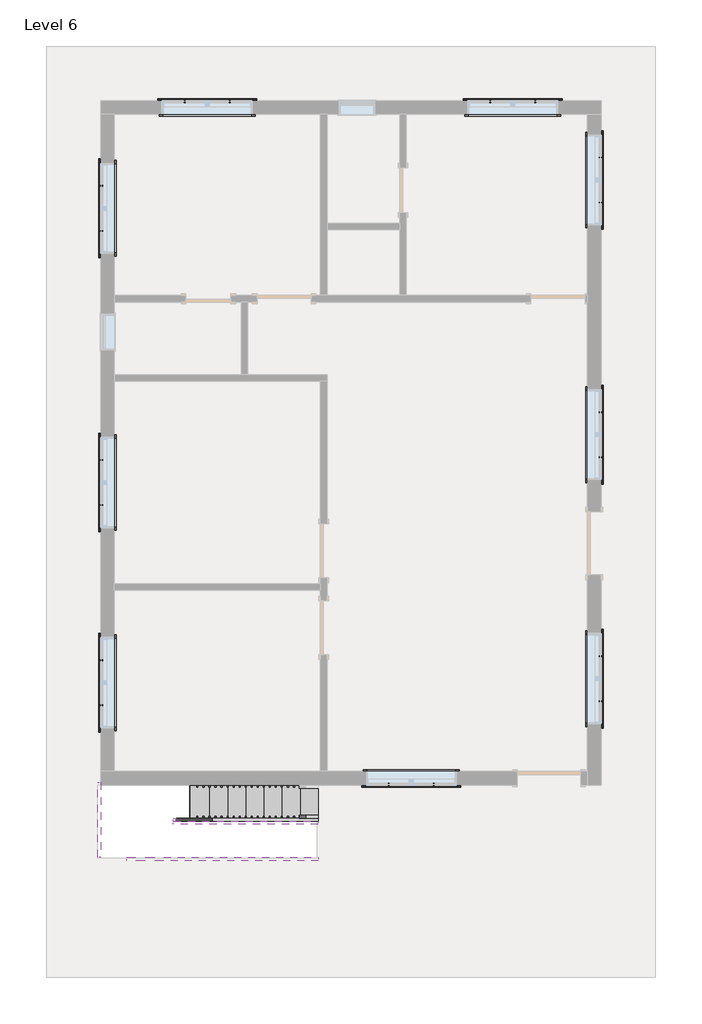
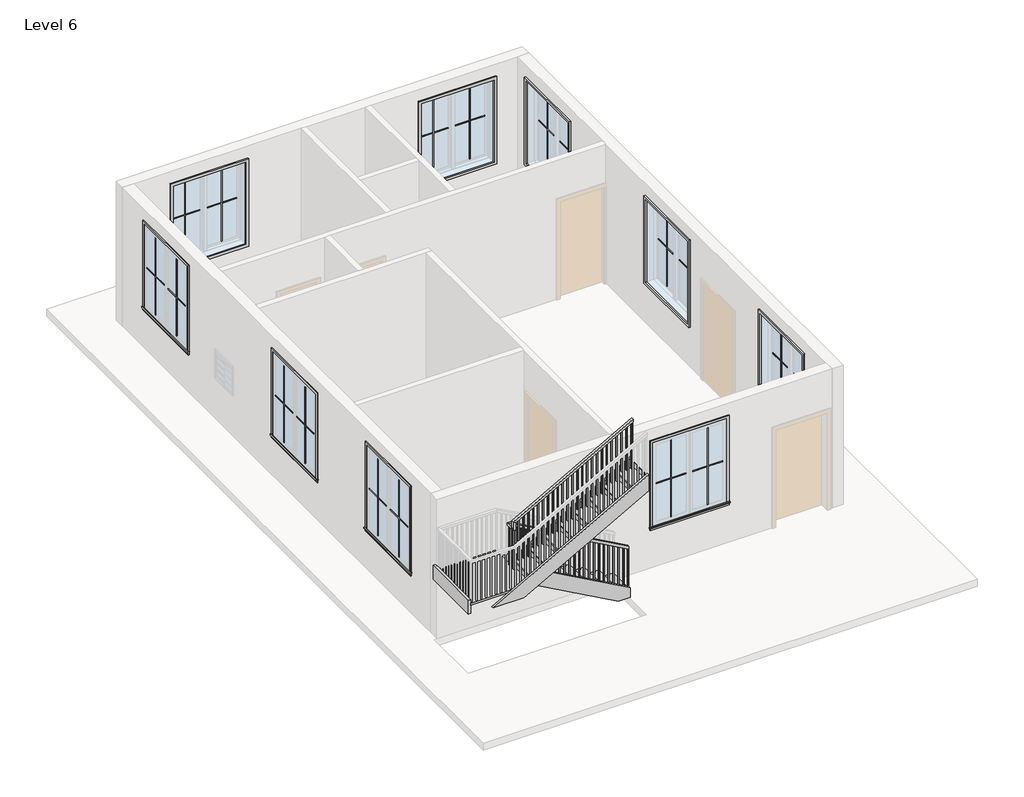
# One storey, part 3 of 3: 36 proxies, 6 members, 1 railing, 1 stair flight.
"""IFC4 building model written with IfcOpenShell, lengths in millimetres."""

from ifc_helpers import new_model, si_unit, frame, origin, place, context, project, spatial, polyline, outline, extrude, faceted_brep, transform, mapped, element, save
from components import muntin_pattern_2x2_muntin_pattern_2x2_f6a80940, muntin_pattern_2x2_muntin_pattern_2x2_09b00a1c, trim_window_exterior_flat_with_sill_698ed857, trim_window_interior_flat_picture_frame_92551a5e, stair_flight_6b4fcaec

model = new_model("IFC4")

# Units and contexts
model_context = context("Model", 3, world=origin())
ifc_project = project(units=[si_unit("LENGTHUNIT", "METRE", prefix="MILLI")], contexts=[model_context])

# Site, building, storey
site = spatial("IfcSite", under=ifc_project)
building = spatial("IfcBuilding", under=site)
storey = spatial("IfcBuildingStorey", under=building, Name="Level 6", Elevation=12801.6)

# Proxies
placement = place(None, origin())
muntin_pattern_2x2_muntin_pattern_2x2_shape = muntin_pattern_2x2_muntin_pattern_2x2_f6a80940(model_context)
element("IfcBuildingElementProxy", 1, Name="Muntin Pattern_2x2 : Muntin Pattern_2x2", ObjectType="Muntin Pattern_2x2 : Muntin Pattern_2x2", at=placement, inside=storey, context=model_context, shape_type="MappedRepresentation", body=[
    mapped(muntin_pattern_2x2_muntin_pattern_2x2_shape, transform((-5453.9948569, -3961.7808037, 13785.85), x_axis=(0.0, 1.0, 0.0), y_axis=(-1.0, 0.0, 0.0), z_axis=(0.0, 0.0, 1.0))),
])
element("IfcBuildingElementProxy", 2, Name="Muntin Pattern_2x2 : Muntin Pattern_2x2", ObjectType="Muntin Pattern_2x2 : Muntin Pattern_2x2", at=placement, inside=storey, context=model_context, shape_type="MappedRepresentation", body=[
    mapped(muntin_pattern_2x2_muntin_pattern_2x2_shape, transform((-5453.9948569, -593.1058037, 13785.85), x_axis=(0.0, 1.0, 0.0), y_axis=(-1.0, 0.0, 0.0), z_axis=(0.0, 0.0, 1.0))),
])
element("IfcBuildingElementProxy", 3, Name="Muntin Pattern_2x2 : Muntin Pattern_2x2", ObjectType="Muntin Pattern_2x2 : Muntin Pattern_2x2", at=placement, inside=storey, context=model_context, shape_type="MappedRepresentation", body=[
    mapped(muntin_pattern_2x2_muntin_pattern_2x2_shape, transform((-5453.9948569, 4023.3441963, 13785.85), x_axis=(0.0, 1.0, 0.0), y_axis=(-1.0, 0.0, 0.0), z_axis=(0.0, 0.0, 1.0))),
])
element("IfcBuildingElementProxy", 4, Name="Muntin Pattern_2x2 : Muntin Pattern_2x2", ObjectType="Muntin Pattern_2x2 : Muntin Pattern_2x2", at=placement, inside=storey, context=model_context, shape_type="MappedRepresentation", body=[
    mapped(muntin_pattern_2x2_muntin_pattern_2x2_shape, transform((2947.0551431, 5258.4191963, 13785.85), x_axis=(0.0, -1.0, 0.0), y_axis=(1.0, 0.0, 0.0), z_axis=(0.0, 0.0, 1.0))),
])
element("IfcBuildingElementProxy", 5, Name="Muntin Pattern_2x2 : Muntin Pattern_2x2", ObjectType="Muntin Pattern_2x2 : Muntin Pattern_2x2", at=placement, inside=storey, context=model_context, shape_type="MappedRepresentation", body=[
    mapped(muntin_pattern_2x2_muntin_pattern_2x2_shape, transform((2947.0551431, 972.1691963, 13785.85), x_axis=(0.0, -1.0, 0.0), y_axis=(1.0, 0.0, 0.0), z_axis=(0.0, 0.0, 1.0))),
])
element("IfcBuildingElementProxy", 6, Name="Muntin Pattern_2x2 : Muntin Pattern_2x2", ObjectType="Muntin Pattern_2x2 : Muntin Pattern_2x2", at=placement, inside=storey, context=model_context, shape_type="MappedRepresentation", body=[
    mapped(muntin_pattern_2x2_muntin_pattern_2x2_shape, transform((2947.0551431, -3136.2808037, 13785.85), x_axis=(0.0, -1.0, 0.0), y_axis=(1.0, 0.0, 0.0), z_axis=(0.0, 0.0, 1.0))),
])
element("IfcBuildingElementProxy", 7, Name="Muntin Pattern_2x2 : Muntin Pattern_2x2", ObjectType="Muntin Pattern_2x2 : Muntin Pattern_2x2", at=placement, inside=storey, context=model_context, shape_type="MappedRepresentation", body=[
    mapped(muntin_pattern_2x2_muntin_pattern_2x2_shape, transform((141.9426431, -5296.8683037, 13785.85), x_axis=(-1.0, 0.0, 0.0), y_axis=(0.0, -1.0, 0.0), z_axis=(0.0, 0.0, 1.0))),
])
element("IfcBuildingElementProxy", 8, Name="Muntin Pattern_2x2 : Muntin Pattern_2x2", ObjectType="Muntin Pattern_2x2 : Muntin Pattern_2x2", at=placement, inside=storey, context=model_context, shape_type="MappedRepresentation", body=[
    mapped(muntin_pattern_2x2_muntin_pattern_2x2_shape, transform((1091.2676431, 6202.9816963, 13785.85), x_axis=(1.0, 0.0, 0.0), y_axis=(0.0, 1.0, 0.0), z_axis=(0.0, 0.0, 1.0))),
])
element("IfcBuildingElementProxy", 9, Name="Muntin Pattern_2x2 : Muntin Pattern_2x2", ObjectType="Muntin Pattern_2x2 : Muntin Pattern_2x2", at=placement, inside=storey, context=model_context, shape_type="MappedRepresentation", body=[
    mapped(muntin_pattern_2x2_muntin_pattern_2x2_shape, transform((-4052.2323569, 6202.9816963, 13785.85), x_axis=(1.0, 0.0, 0.0), y_axis=(0.0, 1.0, 0.0), z_axis=(0.0, 0.0, 1.0))),
])
muntin_pattern_2x2_muntin_pattern_2x2_2_shape = muntin_pattern_2x2_muntin_pattern_2x2_09b00a1c(model_context)
element("IfcBuildingElementProxy", 10, Name="Muntin Pattern_2x2 : Muntin Pattern_2x2", ObjectType="Muntin Pattern_2x2 : Muntin Pattern_2x2", at=placement, inside=storey, context=model_context, shape_type="MappedRepresentation", body=[
    mapped(muntin_pattern_2x2_muntin_pattern_2x2_2_shape, transform((-5453.9948569, -3202.9558037, 13785.85), x_axis=(0.0, -1.0, 0.0), y_axis=(1.0, 0.0, 0.0), z_axis=(0.0, 0.0, 1.0))),
])
element("IfcBuildingElementProxy", 11, Name="Muntin Pattern_2x2 : Muntin Pattern_2x2", ObjectType="Muntin Pattern_2x2 : Muntin Pattern_2x2", at=placement, inside=storey, context=model_context, shape_type="MappedRepresentation", body=[
    mapped(muntin_pattern_2x2_muntin_pattern_2x2_2_shape, transform((-5453.9948569, 165.7191963, 13785.85), x_axis=(0.0, -1.0, 0.0), y_axis=(1.0, 0.0, 0.0), z_axis=(0.0, 0.0, 1.0))),
])
element("IfcBuildingElementProxy", 12, Name="Muntin Pattern_2x2 : Muntin Pattern_2x2", ObjectType="Muntin Pattern_2x2 : Muntin Pattern_2x2", at=placement, inside=storey, context=model_context, shape_type="MappedRepresentation", body=[
    mapped(muntin_pattern_2x2_muntin_pattern_2x2_2_shape, transform((-5453.9948569, 4782.1691963, 13785.85), x_axis=(0.0, -1.0, 0.0), y_axis=(1.0, 0.0, 0.0), z_axis=(0.0, 0.0, 1.0))),
])
element("IfcBuildingElementProxy", 13, Name="Muntin Pattern_2x2 : Muntin Pattern_2x2", ObjectType="Muntin Pattern_2x2 : Muntin Pattern_2x2", at=placement, inside=storey, context=model_context, shape_type="MappedRepresentation", body=[
    mapped(muntin_pattern_2x2_muntin_pattern_2x2_2_shape, transform((2947.0551431, 4499.5941963, 13785.85), x_axis=(0.0, 1.0, 0.0), y_axis=(-1.0, 0.0, 0.0), z_axis=(0.0, 0.0, 1.0))),
])
element("IfcBuildingElementProxy", 14, Name="Muntin Pattern_2x2 : Muntin Pattern_2x2", ObjectType="Muntin Pattern_2x2 : Muntin Pattern_2x2", at=placement, inside=storey, context=model_context, shape_type="MappedRepresentation", body=[
    mapped(muntin_pattern_2x2_muntin_pattern_2x2_2_shape, transform((2947.0551431, 213.3441963, 13785.85), x_axis=(0.0, 1.0, 0.0), y_axis=(-1.0, 0.0, 0.0), z_axis=(0.0, 0.0, 1.0))),
])
element("IfcBuildingElementProxy", 15, Name="Muntin Pattern_2x2 : Muntin Pattern_2x2", ObjectType="Muntin Pattern_2x2 : Muntin Pattern_2x2", at=placement, inside=storey, context=model_context, shape_type="MappedRepresentation", body=[
    mapped(muntin_pattern_2x2_muntin_pattern_2x2_2_shape, transform((2947.0551431, -3895.1058037, 13785.85), x_axis=(0.0, 1.0, 0.0), y_axis=(-1.0, 0.0, 0.0), z_axis=(0.0, 0.0, 1.0))),
])
element("IfcBuildingElementProxy", 16, Name="Muntin Pattern_2x2 : Muntin Pattern_2x2", ObjectType="Muntin Pattern_2x2 : Muntin Pattern_2x2", at=placement, inside=storey, context=model_context, shape_type="MappedRepresentation", body=[
    mapped(muntin_pattern_2x2_muntin_pattern_2x2_2_shape, transform((-616.8823569, -5296.8683037, 13785.85), x_axis=(1.0, 0.0, 0.0), y_axis=(0.0, 1.0, 0.0), z_axis=(0.0, 0.0, 1.0))),
])
element("IfcBuildingElementProxy", 17, Name="Muntin Pattern_2x2 : Muntin Pattern_2x2", ObjectType="Muntin Pattern_2x2 : Muntin Pattern_2x2", at=placement, inside=storey, context=model_context, shape_type="MappedRepresentation", body=[
    mapped(muntin_pattern_2x2_muntin_pattern_2x2_2_shape, transform((1850.0926431, 6202.9816963, 13785.85), x_axis=(-1.0, 0.0, 0.0), y_axis=(0.0, -1.0, 0.0), z_axis=(0.0, 0.0, 1.0))),
])
element("IfcBuildingElementProxy", 18, Name="Muntin Pattern_2x2 : Muntin Pattern_2x2", ObjectType="Muntin Pattern_2x2 : Muntin Pattern_2x2", at=placement, inside=storey, context=model_context, shape_type="MappedRepresentation", body=[
    mapped(muntin_pattern_2x2_muntin_pattern_2x2_2_shape, transform((-3293.4073569, 6202.9816963, 13785.85), x_axis=(-1.0, 0.0, 0.0), y_axis=(0.0, -1.0, 0.0), z_axis=(0.0, 0.0, 1.0))),
])
trim_window_exterior_flat_with_sill_shape = trim_window_exterior_flat_with_sill_698ed857(model_context)
element("IfcBuildingElementProxy", 19, Name="Trim-Window-Exterior-Flat : with Sill", ObjectType="Trim-Window-Exterior-Flat : with Sill", at=placement, inside=storey, context=model_context, shape_type="MappedRepresentation", body=[
    mapped(trim_window_exterior_flat_with_sill_shape, transform((-5463.5198569, -3582.3683037, 15544.8), x_axis=(0.0, -1.0, 0.0), y_axis=(0.0, 0.0, 1.0), z_axis=(-1.0, 0.0, 0.0))),
])
element("IfcBuildingElementProxy", 20, Name="Trim-Window-Exterior-Flat : with Sill", ObjectType="Trim-Window-Exterior-Flat : with Sill", at=placement, inside=storey, context=model_context, shape_type="MappedRepresentation", body=[
    mapped(trim_window_exterior_flat_with_sill_shape, transform((-5463.5198569, -213.6933037, 15544.8), x_axis=(0.0, -1.0, 0.0), y_axis=(0.0, 0.0, 1.0), z_axis=(-1.0, 0.0, 0.0))),
])
element("IfcBuildingElementProxy", 21, Name="Trim-Window-Exterior-Flat : with Sill", ObjectType="Trim-Window-Exterior-Flat : with Sill", at=placement, inside=storey, context=model_context, shape_type="MappedRepresentation", body=[
    mapped(trim_window_exterior_flat_with_sill_shape, transform((-5463.5198569, 4402.7566963, 15544.8), x_axis=(0.0, -1.0, 0.0), y_axis=(0.0, 0.0, 1.0), z_axis=(-1.0, 0.0, 0.0))),
])
element("IfcBuildingElementProxy", 22, Name="Trim-Window-Exterior-Flat : with Sill", ObjectType="Trim-Window-Exterior-Flat : with Sill", at=placement, inside=storey, context=model_context, shape_type="MappedRepresentation", body=[
    mapped(trim_window_exterior_flat_with_sill_shape, transform((2956.5801431, 4879.0066963, 15544.8), x_axis=(0.0, 1.0, 0.0), y_axis=(0.0, 0.0, 1.0), z_axis=(1.0, 0.0, 0.0))),
])
element("IfcBuildingElementProxy", 23, Name="Trim-Window-Exterior-Flat : with Sill", ObjectType="Trim-Window-Exterior-Flat : with Sill", at=placement, inside=storey, context=model_context, shape_type="MappedRepresentation", body=[
    mapped(trim_window_exterior_flat_with_sill_shape, transform((2956.5801431, 592.7566963, 15544.8), x_axis=(0.0, 1.0, 0.0), y_axis=(0.0, 0.0, 1.0), z_axis=(1.0, 0.0, 0.0))),
])
element("IfcBuildingElementProxy", 24, Name="Trim-Window-Exterior-Flat : with Sill", ObjectType="Trim-Window-Exterior-Flat : with Sill", at=placement, inside=storey, context=model_context, shape_type="MappedRepresentation", body=[
    mapped(trim_window_exterior_flat_with_sill_shape, transform((2956.5801431, -3515.6933037, 15544.8), x_axis=(0.0, 1.0, 0.0), y_axis=(0.0, 0.0, 1.0), z_axis=(1.0, 0.0, 0.0))),
])
element("IfcBuildingElementProxy", 25, Name="Trim-Window-Exterior-Flat : with Sill", ObjectType="Trim-Window-Exterior-Flat : with Sill", at=placement, inside=storey, context=model_context, shape_type="MappedRepresentation", body=[
    mapped(trim_window_exterior_flat_with_sill_shape, transform((-237.4698569, -5306.3933037, 15544.8), x_axis=(1.0, 0.0, 0.0), y_axis=(0.0, 0.0, 1.0), z_axis=(0.0, -1.0, 0.0))),
])
element("IfcBuildingElementProxy", 26, Name="Trim-Window-Exterior-Flat : with Sill", ObjectType="Trim-Window-Exterior-Flat : with Sill", at=placement, inside=storey, context=model_context, shape_type="MappedRepresentation", body=[
    mapped(trim_window_exterior_flat_with_sill_shape, transform((1470.6801431, 6212.5066963, 15544.8), x_axis=(-1.0, 0.0, 0.0), y_axis=(0.0, 0.0, 1.0), z_axis=(0.0, 1.0, 0.0))),
])
element("IfcBuildingElementProxy", 27, Name="Trim-Window-Exterior-Flat : with Sill", ObjectType="Trim-Window-Exterior-Flat : with Sill", at=placement, inside=storey, context=model_context, shape_type="MappedRepresentation", body=[
    mapped(trim_window_exterior_flat_with_sill_shape, transform((-3672.8198569, 6212.5066963, 15544.8), x_axis=(-1.0, 0.0, 0.0), y_axis=(0.0, 0.0, 1.0), z_axis=(0.0, 1.0, 0.0))),
])
trim_window_interior_flat_picture_frame_shape = trim_window_interior_flat_picture_frame_92551a5e(model_context)
element("IfcBuildingElementProxy", 28, Name="Trim-Window-Interior-Flat : Picture Frame", ObjectType="Trim-Window-Interior-Flat : Picture Frame", at=placement, inside=storey, context=model_context, shape_type="MappedRepresentation", body=[
    mapped(trim_window_interior_flat_picture_frame_shape, transform((-5234.9198569, -3582.3683037, 15544.8), x_axis=(0.0, 1.0, 0.0), y_axis=(0.0, 0.0, 1.0), z_axis=(1.0, 0.0, 0.0))),
])
element("IfcBuildingElementProxy", 29, Name="Trim-Window-Interior-Flat : Picture Frame", ObjectType="Trim-Window-Interior-Flat : Picture Frame", at=placement, inside=storey, context=model_context, shape_type="MappedRepresentation", body=[
    mapped(trim_window_interior_flat_picture_frame_shape, transform((-5234.9198569, -213.6933037, 15544.8), x_axis=(0.0, 1.0, 0.0), y_axis=(0.0, 0.0, 1.0), z_axis=(1.0, 0.0, 0.0))),
])
element("IfcBuildingElementProxy", 30, Name="Trim-Window-Interior-Flat : Picture Frame", ObjectType="Trim-Window-Interior-Flat : Picture Frame", at=placement, inside=storey, context=model_context, shape_type="MappedRepresentation", body=[
    mapped(trim_window_interior_flat_picture_frame_shape, transform((-5234.9198569, 4402.7566963, 15544.8), x_axis=(0.0, 1.0, 0.0), y_axis=(0.0, 0.0, 1.0), z_axis=(1.0, 0.0, 0.0))),
])
element("IfcBuildingElementProxy", 31, Name="Trim-Window-Interior-Flat : Picture Frame", ObjectType="Trim-Window-Interior-Flat : Picture Frame", at=placement, inside=storey, context=model_context, shape_type="MappedRepresentation", body=[
    mapped(trim_window_interior_flat_picture_frame_shape, transform((2727.9801431, 4879.0066963, 15544.8), x_axis=(0.0, -1.0, 0.0), y_axis=(0.0, 0.0, 1.0), z_axis=(-1.0, 0.0, 0.0))),
])
element("IfcBuildingElementProxy", 32, Name="Trim-Window-Interior-Flat : Picture Frame", ObjectType="Trim-Window-Interior-Flat : Picture Frame", at=placement, inside=storey, context=model_context, shape_type="MappedRepresentation", body=[
    mapped(trim_window_interior_flat_picture_frame_shape, transform((2727.9801431, 592.7566963, 15544.8), x_axis=(0.0, -1.0, 0.0), y_axis=(0.0, 0.0, 1.0), z_axis=(-1.0, 0.0, 0.0))),
])
element("IfcBuildingElementProxy", 33, Name="Trim-Window-Interior-Flat : Picture Frame", ObjectType="Trim-Window-Interior-Flat : Picture Frame", at=placement, inside=storey, context=model_context, shape_type="MappedRepresentation", body=[
    mapped(trim_window_interior_flat_picture_frame_shape, transform((2727.9801431, -3515.6933037, 15544.8), x_axis=(0.0, -1.0, 0.0), y_axis=(0.0, 0.0, 1.0), z_axis=(-1.0, 0.0, 0.0))),
])
element("IfcBuildingElementProxy", 34, Name="Trim-Window-Interior-Flat : Picture Frame", ObjectType="Trim-Window-Interior-Flat : Picture Frame", at=placement, inside=storey, context=model_context, shape_type="MappedRepresentation", body=[
    mapped(trim_window_interior_flat_picture_frame_shape, transform((-237.4698569, -5077.7933037, 15544.8), x_axis=(-1.0, 0.0, 0.0), y_axis=(0.0, 0.0, 1.0), z_axis=(0.0, 1.0, 0.0))),
])
element("IfcBuildingElementProxy", 35, Name="Trim-Window-Interior-Flat : Picture Frame", ObjectType="Trim-Window-Interior-Flat : Picture Frame", at=placement, inside=storey, context=model_context, shape_type="MappedRepresentation", body=[
    mapped(trim_window_interior_flat_picture_frame_shape, transform((1470.6801431, 5983.9066963, 15544.8), x_axis=(1.0, 0.0, 0.0), y_axis=(0.0, 0.0, 1.0), z_axis=(0.0, -1.0, 0.0))),
])
element("IfcBuildingElementProxy", 36, Name="Trim-Window-Interior-Flat : Picture Frame", ObjectType="Trim-Window-Interior-Flat : Picture Frame", at=placement, inside=storey, context=model_context, shape_type="MappedRepresentation", body=[
    mapped(trim_window_interior_flat_picture_frame_shape, transform((-3672.8198569, 5983.9066963, 15544.8), x_axis=(1.0, 0.0, 0.0), y_axis=(0.0, 0.0, 1.0), z_axis=(0.0, -1.0, 0.0))),
])

# Members
element("IfcMember", 37, ObjectType="Stringer - 2\" Width", at=placement, inside=storey, context=model_context, shape_type="SweptSolid", body=[
    extrude(outline(polyline([(12801.6, -1805.9198569), (13009.1983948, -1805.9198569), (14335.6428392, -4193.5198569), (13986.9641651, -4193.5198569), (12801.6, -2059.8643597), (12801.6, -1805.9198569)])), frame((0.0, -5915.9933037, 0.0), z_axis=(0.0, 1.0, 0.0), x_axis=(0.0, 0.0, 1.0)), (0.0, 0.0, 1.0), 50.8),
])
element("IfcMember", 38, ObjectType="Stringer - 2\" Width", at=placement, inside=storey, context=model_context, shape_type="SweptSolid", body=[
    extrude(outline(polyline([(-4244.3198569, -5865.1933037), (-4193.5198569, -5865.1933037), (-4193.5198569, -5915.9933037), (-4244.3198569, -5915.9933037), (-4244.3198569, -5865.1933037)])), frame((0.0, 0.0, 14097.0), z_axis=(0.0, 0.0, 1.0), x_axis=(1.0, 0.0, 0.0)), (0.0, 0.0, 1.0), 304.8),
])
element("IfcMember", 39, ObjectType="Stringer - 2\" Width", at=placement, inside=storey, context=model_context, shape_type="SweptSolid", body=[
    extrude(outline(polyline([(14533.1983948, -4244.3198569), (14184.5197207, -4244.3198569), (15539.1863873, -1805.9198569), (15887.8650614, -1805.9198569), (14533.1983948, -4244.3198569)])), frame((0.0, -5966.7933037, 0.0), z_axis=(0.0, 1.0, 0.0), x_axis=(0.0, 0.0, 1.0)), (0.0, 0.0, 1.0), 50.8),
])
element("IfcMember", 40, ObjectType="Stringer - 2\" Width", at=placement, inside=storey, context=model_context, shape_type="SweptSolid", body=[
    extrude(outline(polyline([(12801.6, -1805.9198569), (13009.1983948, -1805.9198569), (14401.8, -4312.6027463), (14401.8, -4940.2243597), (12801.6, -2059.8643597), (12801.6, -1805.9198569)])), frame((0.0, -5306.3933037, 0.0), z_axis=(0.0, 1.0, 0.0), x_axis=(0.0, 0.0, 1.0)), (0.0, 0.0, 1.0), 50.8),
])
element("IfcMember", 41, ObjectType="Stringer - 2\" Width", at=placement, inside=storey, context=model_context, shape_type="SweptSolid", body=[
    extrude(outline(polyline([(-5514.3198569, -5255.5933037), (-5463.5198569, -5255.5933037), (-5463.5198569, -6525.5933037), (-5514.3198569, -6525.5933037), (-5514.3198569, -5255.5933037)])), frame((0.0, 0.0, 14097.0), z_axis=(0.0, 0.0, 1.0), x_axis=(1.0, 0.0, 0.0)), (0.0, 0.0, 1.0), 304.8),
])
element("IfcMember", 42, ObjectType="Stringer - 2\" Width", at=placement, inside=storey, context=model_context, shape_type="SweptSolid", body=[
    extrude(outline(polyline([(14097.0, -4401.8553541), (15539.1863873, -1805.9198569), (15887.8650614, -1805.9198569), (14097.0, -5029.4769675), (14097.0, -4401.8553541)])), frame((0.0, -6576.3933037, 0.0), z_axis=(0.0, 1.0, 0.0), x_axis=(0.0, 0.0, 1.0)), (0.0, 0.0, 1.0), 50.8),
])

# Railing
element("IfcRailing", 43, ObjectType="Handrail - Rectangular", at=placement, inside=storey, context=model_context, shape_type="SolidModel", body=[
    faceted_brep([(-1805.9198569, -5865.1933037, 13885.3333333), (-1805.9198569, -5865.1933037, 13827.220221), (-1805.9198569, -5814.3933037, 13827.220221), (-1805.9198569, -5814.3933037, 13885.3333333), (-4168.1198569, -5865.1933037, 15197.6666667), (-4218.9198569, -5865.1933037, 15167.7757765), (-4218.9198569, -5814.3933037, 15167.7757765), (-4168.1198569, -5814.3933037, 15197.6666667), (-4168.1198569, -5865.1933037, 15240.0), (-4218.9198569, -5865.1933037, 15189.2), (-4218.9198569, -5814.3933037, 15189.2), (-4168.1198569, -5814.3933037, 15240.0), (-4244.3198569, -5865.1933037, 15240.0), (-4244.3198569, -5865.1933037, 15189.2), (-4295.1198569, -5814.3933037, 15189.2), (-4295.1198569, -5814.3933037, 15240.0), (-4244.3198569, -5941.3933037, 15240.0), (-4244.3198569, -5941.3933037, 15189.2), (-4295.1198569, -5941.3933037, 15189.2), (-4295.1198569, -5941.3933037, 15240.0), (-4244.3198569, -5966.7933037, 15240.0), (-4295.1198569, -5966.7933037, 15240.0), (-4295.1198569, -6017.5933037, 15189.2), (-4244.3198569, -6017.5933037, 15189.2)], [[[0, 1, 2, 3]], [[1, 0, 4, 5]], [[2, 1, 5, 6]], [[3, 2, 6, 7]], [[0, 3, 7, 4]], [[5, 4, 8, 9]], [[6, 5, 9, 10]], [[7, 6, 10, 11]], [[4, 7, 11, 8]], [[9, 8, 12, 13]], [[10, 9, 13, 14]], [[11, 10, 14, 15]], [[8, 11, 15, 12]], [[13, 12, 16, 17]], [[14, 13, 17, 18]], [[15, 14, 18, 19]], [[12, 15, 19, 16]], [[20, 21, 22, 23]], [[17, 16, 20, 23]], [[18, 17, 23, 22]], [[19, 18, 22, 21]], [[16, 19, 21, 20]]]),
    faceted_brep([(-4244.3198569, -5966.7933037, 15240.0), (-4244.3198569, -6017.5933037, 15189.2), (-4295.1198569, -6017.5933037, 15189.2), (-4295.1198569, -5966.7933037, 15240.0), (-4244.3198569, -5966.7933037, 15351.220221), (-4295.1198569, -5966.7933037, 15381.1111111), (-4295.1198569, -6017.5933037, 15381.1111111), (-4244.3198569, -6017.5933037, 15351.220221)], [[[0, 1, 2, 3]], [[4, 5, 6, 7]], [[1, 0, 4, 7]], [[2, 1, 7, 6]], [[3, 2, 6, 5]], [[0, 3, 5, 4]]]),
    faceted_brep([(-4295.1198569, -5966.7933037, 15381.1111111), (-4244.3198569, -5966.7933037, 15351.220221), (-4244.3198569, -6017.5933037, 15351.220221), (-4295.1198569, -6017.5933037, 15381.1111111), (-1805.9198569, -5966.7933037, 16764.0), (-1805.9198569, -6017.5933037, 16764.0), (-1805.9198569, -6017.5933037, 16705.8868876), (-1805.9198569, -5966.7933037, 16705.8868876)], [[[0, 1, 2, 3]], [[4, 5, 6, 7]], [[1, 0, 4, 7]], [[2, 1, 7, 6]], [[3, 2, 6, 5]], [[0, 3, 5, 4]]]),
    extrude(outline(polyline([(16686.4841099, -1840.8448569), (15680.2666667, -1840.8448569), (15680.2666667, -1821.7948569), (16697.0674432, -1821.7948569), (16686.4841099, -1840.8448569)])), frame((0.0, -6001.7183037, 0.0), z_axis=(0.0, 1.0, 0.0), x_axis=(0.0, 0.0, 1.0)), (0.0, 0.0, 1.0), 19.05),
    extrude(outline(polyline([(16630.0396654, -1942.4448569), (15680.2666667, -1942.4448569), (15680.2666667, -1923.3948569), (16640.6229988, -1923.3948569), (16630.0396654, -1942.4448569)])), frame((0.0, -6001.7183037, 0.0), z_axis=(0.0, 1.0, 0.0), x_axis=(0.0, 0.0, 1.0)), (0.0, 0.0, 1.0), 19.05),
    extrude(outline(polyline([(16573.595221, -2044.0448569), (15680.2666667, -2044.0448569), (15680.2666667, -2024.9948569), (16584.1785543, -2024.9948569), (16573.595221, -2044.0448569)])), frame((0.0, -6001.7183037, 0.0), z_axis=(0.0, 1.0, 0.0), x_axis=(0.0, 0.0, 1.0)), (0.0, 0.0, 1.0), 19.05),
    extrude(outline(polyline([(16517.1507765, -2145.6448569), (15510.9333333, -2145.6448569), (15510.9333333, -2126.5948569), (16527.7341099, -2126.5948569), (16517.1507765, -2145.6448569)])), frame((0.0, -6001.7183037, 0.0), z_axis=(0.0, 1.0, 0.0), x_axis=(0.0, 0.0, 1.0)), (0.0, 0.0, 1.0), 19.05),
    extrude(outline(polyline([(16460.7063321, -2247.2448569), (15510.9333333, -2247.2448569), (15510.9333333, -2228.1948569), (16471.2896654, -2228.1948569), (16460.7063321, -2247.2448569)])), frame((0.0, -6001.7183037, 0.0), z_axis=(0.0, 1.0, 0.0), x_axis=(0.0, 0.0, 1.0)), (0.0, 0.0, 1.0), 19.05),
    extrude(outline(polyline([(16404.2618876, -2348.8448569), (15510.9333333, -2348.8448569), (15510.9333333, -2329.7948569), (16414.845221, -2329.7948569), (16404.2618876, -2348.8448569)])), frame((0.0, -6001.7183037, 0.0), z_axis=(0.0, 1.0, 0.0), x_axis=(0.0, 0.0, 1.0)), (0.0, 0.0, 1.0), 19.05),
    extrude(outline(polyline([(16347.8174432, -2450.4448569), (15341.6, -2450.4448569), (15341.6, -2431.3948569), (16358.4007765, -2431.3948569), (16347.8174432, -2450.4448569)])), frame((0.0, -6001.7183037, 0.0), z_axis=(0.0, 1.0, 0.0), x_axis=(0.0, 0.0, 1.0)), (0.0, 0.0, 1.0), 19.05),
    extrude(outline(polyline([(16291.3729988, -2552.0448569), (15341.6, -2552.0448569), (15341.6, -2532.9948569), (16301.9563321, -2532.9948569), (16291.3729988, -2552.0448569)])), frame((0.0, -6001.7183037, 0.0), z_axis=(0.0, 1.0, 0.0), x_axis=(0.0, 0.0, 1.0)), (0.0, 0.0, 1.0), 19.05),
    extrude(outline(polyline([(16234.9285543, -2653.6448569), (15341.6, -2653.6448569), (15341.6, -2634.5948569), (16245.5118876, -2634.5948569), (16234.9285543, -2653.6448569)])), frame((0.0, -6001.7183037, 0.0), z_axis=(0.0, 1.0, 0.0), x_axis=(0.0, 0.0, 1.0)), (0.0, 0.0, 1.0), 19.05),
    extrude(outline(polyline([(16178.4841099, -2755.2448569), (15172.2666667, -2755.2448569), (15172.2666667, -2736.1948569), (16189.0674432, -2736.1948569), (16178.4841099, -2755.2448569)])), frame((0.0, -6001.7183037, 0.0), z_axis=(0.0, 1.0, 0.0), x_axis=(0.0, 0.0, 1.0)), (0.0, 0.0, 1.0), 19.05),
    extrude(outline(polyline([(16122.0396654, -2856.8448569), (15172.2666667, -2856.8448569), (15172.2666667, -2837.7948569), (16132.6229988, -2837.7948569), (16122.0396654, -2856.8448569)])), frame((0.0, -6001.7183037, 0.0), z_axis=(0.0, 1.0, 0.0), x_axis=(0.0, 0.0, 1.0)), (0.0, 0.0, 1.0), 19.05),
    extrude(outline(polyline([(16065.595221, -2958.4448569), (15172.2666667, -2958.4448569), (15172.2666667, -2939.3948569), (16076.1785543, -2939.3948569), (16065.595221, -2958.4448569)])), frame((0.0, -6001.7183037, 0.0), z_axis=(0.0, 1.0, 0.0), x_axis=(0.0, 0.0, 1.0)), (0.0, 0.0, 1.0), 19.05),
    extrude(outline(polyline([(16009.1507765, -3060.0448569), (15002.9333333, -3060.0448569), (15002.9333333, -3040.9948569), (16019.7341099, -3040.9948569), (16009.1507765, -3060.0448569)])), frame((0.0, -6001.7183037, 0.0), z_axis=(0.0, 1.0, 0.0), x_axis=(0.0, 0.0, 1.0)), (0.0, 0.0, 1.0), 19.05),
    extrude(outline(polyline([(15952.7063321, -3161.6448569), (15002.9333333, -3161.6448569), (15002.9333333, -3142.5948569), (15963.2896654, -3142.5948569), (15952.7063321, -3161.6448569)])), frame((0.0, -6001.7183037, 0.0), z_axis=(0.0, 1.0, 0.0), x_axis=(0.0, 0.0, 1.0)), (0.0, 0.0, 1.0), 19.05),
    extrude(outline(polyline([(15896.2618876, -3263.2448569), (15002.9333333, -3263.2448569), (15002.9333333, -3244.1948569), (15906.845221, -3244.1948569), (15896.2618876, -3263.2448569)])), frame((0.0, -6001.7183037, 0.0), z_axis=(0.0, 1.0, 0.0), x_axis=(0.0, 0.0, 1.0)), (0.0, 0.0, 1.0), 19.05),
    extrude(outline(polyline([(15839.8174432, -3364.8448569), (14833.6, -3364.8448569), (14833.6, -3345.7948569), (15850.4007765, -3345.7948569), (15839.8174432, -3364.8448569)])), frame((0.0, -6001.7183037, 0.0), z_axis=(0.0, 1.0, 0.0), x_axis=(0.0, 0.0, 1.0)), (0.0, 0.0, 1.0), 19.05),
    extrude(outline(polyline([(15783.3729988, -3466.4448569), (14833.6, -3466.4448569), (14833.6, -3447.3948569), (15793.9563321, -3447.3948569), (15783.3729988, -3466.4448569)])), frame((0.0, -6001.7183037, 0.0), z_axis=(0.0, 1.0, 0.0), x_axis=(0.0, 0.0, 1.0)), (0.0, 0.0, 1.0), 19.05),
    extrude(outline(polyline([(15726.9285543, -3568.0448569), (14833.6, -3568.0448569), (14833.6, -3548.9948569), (15737.5118876, -3548.9948569), (15726.9285543, -3568.0448569)])), frame((0.0, -6001.7183037, 0.0), z_axis=(0.0, 1.0, 0.0), x_axis=(0.0, 0.0, 1.0)), (0.0, 0.0, 1.0), 19.05),
    extrude(outline(polyline([(15670.4841099, -3669.6448569), (14664.2666667, -3669.6448569), (14664.2666667, -3650.5948569), (15681.0674432, -3650.5948569), (15670.4841099, -3669.6448569)])), frame((0.0, -6001.7183037, 0.0), z_axis=(0.0, 1.0, 0.0), x_axis=(0.0, 0.0, 1.0)), (0.0, 0.0, 1.0), 19.05),
    extrude(outline(polyline([(15614.0396654, -3771.2448569), (14664.2666667, -3771.2448569), (14664.2666667, -3752.1948569), (15624.6229988, -3752.1948569), (15614.0396654, -3771.2448569)])), frame((0.0, -6001.7183037, 0.0), z_axis=(0.0, 1.0, 0.0), x_axis=(0.0, 0.0, 1.0)), (0.0, 0.0, 1.0), 19.05),
    extrude(outline(polyline([(15557.595221, -3872.8448569), (14664.2666667, -3872.8448569), (14664.2666667, -3853.7948569), (15568.1785543, -3853.7948569), (15557.595221, -3872.8448569)])), frame((0.0, -6001.7183037, 0.0), z_axis=(0.0, 1.0, 0.0), x_axis=(0.0, 0.0, 1.0)), (0.0, 0.0, 1.0), 19.05),
    extrude(outline(polyline([(15501.1507765, -3974.4448569), (14494.9333333, -3974.4448569), (14494.9333333, -3955.3948569), (15511.7341099, -3955.3948569), (15501.1507765, -3974.4448569)])), frame((0.0, -6001.7183037, 0.0), z_axis=(0.0, 1.0, 0.0), x_axis=(0.0, 0.0, 1.0)), (0.0, 0.0, 1.0), 19.05),
    extrude(outline(polyline([(15444.7063321, -4076.0448569), (14494.9333333, -4076.0448569), (14494.9333333, -4056.9948569), (15455.2896654, -4056.9948569), (15444.7063321, -4076.0448569)])), frame((0.0, -6001.7183037, 0.0), z_axis=(0.0, 1.0, 0.0), x_axis=(0.0, 0.0, 1.0)), (0.0, 0.0, 1.0), 19.05),
    extrude(outline(polyline([(15388.2618876, -4177.6448569), (14494.9333333, -4177.6448569), (14494.9333333, -4158.5948569), (15398.845221, -4158.5948569), (15388.2618876, -4177.6448569)])), frame((0.0, -6001.7183037, 0.0), z_axis=(0.0, 1.0, 0.0), x_axis=(0.0, 0.0, 1.0)), (0.0, 0.0, 1.0), 19.05),
    extrude(outline(polyline([(-4260.1948569, -5931.8683037), (-4260.1948569, -5950.9183037), (-4279.2448569, -5950.9183037), (-4279.2448569, -5931.8683037), (-4260.1948569, -5931.8683037)])), frame((0.0, 0.0, 14325.6), z_axis=(0.0, 0.0, 1.0), x_axis=(1.0, 0.0, 0.0)), (0.0, 0.0, 1.0), 863.6),
    extrude(outline(polyline([(-4234.7948569, -5849.3183037), (-4253.8448569, -5849.3183037), (-4253.8448569, -5830.2683037), (-4234.7948569, -5830.2683037), (-4234.7948569, -5849.3183037)])), frame((0.0, 0.0, 14325.6), z_axis=(0.0, 0.0, 1.0), x_axis=(1.0, 0.0, 0.0)), (0.0, 0.0, 1.0), 863.6),
    extrude(outline(polyline([(15130.7341099, -4152.2448569), (14156.2666667, -4152.2448569), (14156.2666667, -4133.1948569), (15120.1507765, -4133.1948569), (15130.7341099, -4152.2448569)])), frame((0.0, -5849.3183037, 0.0), z_axis=(0.0, 1.0, 0.0), x_axis=(0.0, 0.0, 1.0)), (0.0, 0.0, 1.0), 19.05),
    extrude(outline(polyline([(15074.2896654, -4050.6448569), (14156.2666667, -4050.6448569), (14156.2666667, -4031.5948569), (15063.7063321, -4031.5948569), (15074.2896654, -4050.6448569)])), frame((0.0, -5849.3183037, 0.0), z_axis=(0.0, 1.0, 0.0), x_axis=(0.0, 0.0, 1.0)), (0.0, 0.0, 1.0), 19.05),
    extrude(outline(polyline([(15017.845221, -3949.0448569), (14156.2666667, -3949.0448569), (14156.2666667, -3929.9948569), (15007.2618876, -3929.9948569), (15017.845221, -3949.0448569)])), frame((0.0, -5849.3183037, 0.0), z_axis=(0.0, 1.0, 0.0), x_axis=(0.0, 0.0, 1.0)), (0.0, 0.0, 1.0), 19.05),
    extrude(outline(polyline([(14961.4007765, -3847.4448569), (13986.9333333, -3847.4448569), (13986.9333333, -3828.3948569), (14950.8174432, -3828.3948569), (14961.4007765, -3847.4448569)])), frame((0.0, -5849.3183037, 0.0), z_axis=(0.0, 1.0, 0.0), x_axis=(0.0, 0.0, 1.0)), (0.0, 0.0, 1.0), 19.05),
    extrude(outline(polyline([(14904.9563321, -3745.8448569), (13986.9333333, -3745.8448569), (13986.9333333, -3726.7948569), (14894.3729988, -3726.7948569), (14904.9563321, -3745.8448569)])), frame((0.0, -5849.3183037, 0.0), z_axis=(0.0, 1.0, 0.0), x_axis=(0.0, 0.0, 1.0)), (0.0, 0.0, 1.0), 19.05),
    extrude(outline(polyline([(14848.5118876, -3644.2448569), (13986.9333333, -3644.2448569), (13986.9333333, -3625.1948569), (14837.9285543, -3625.1948569), (14848.5118876, -3644.2448569)])), frame((0.0, -5849.3183037, 0.0), z_axis=(0.0, 1.0, 0.0), x_axis=(0.0, 0.0, 1.0)), (0.0, 0.0, 1.0), 19.05),
    extrude(outline(polyline([(14792.0674432, -3542.6448569), (13817.6, -3542.6448569), (13817.6, -3523.5948569), (14781.4841099, -3523.5948569), (14792.0674432, -3542.6448569)])), frame((0.0, -5849.3183037, 0.0), z_axis=(0.0, 1.0, 0.0), x_axis=(0.0, 0.0, 1.0)), (0.0, 0.0, 1.0), 19.05),
    extrude(outline(polyline([(14735.6229988, -3441.0448569), (13817.6, -3441.0448569), (13817.6, -3421.9948569), (14725.0396654, -3421.9948569), (14735.6229988, -3441.0448569)])), frame((0.0, -5849.3183037, 0.0), z_axis=(0.0, 1.0, 0.0), x_axis=(0.0, 0.0, 1.0)), (0.0, 0.0, 1.0), 19.05),
    extrude(outline(polyline([(14679.1785543, -3339.4448569), (13817.6, -3339.4448569), (13817.6, -3320.3948569), (14668.595221, -3320.3948569), (14679.1785543, -3339.4448569)])), frame((0.0, -5849.3183037, 0.0), z_axis=(0.0, 1.0, 0.0), x_axis=(0.0, 0.0, 1.0)), (0.0, 0.0, 1.0), 19.05),
    extrude(outline(polyline([(14622.7341099, -3237.8448569), (13648.2666667, -3237.8448569), (13648.2666667, -3218.7948569), (14612.1507765, -3218.7948569), (14622.7341099, -3237.8448569)])), frame((0.0, -5849.3183037, 0.0), z_axis=(0.0, 1.0, 0.0), x_axis=(0.0, 0.0, 1.0)), (0.0, 0.0, 1.0), 19.05),
    extrude(outline(polyline([(14566.2896654, -3136.2448569), (13648.2666667, -3136.2448569), (13648.2666667, -3117.1948569), (14555.7063321, -3117.1948569), (14566.2896654, -3136.2448569)])), frame((0.0, -5849.3183037, 0.0), z_axis=(0.0, 1.0, 0.0), x_axis=(0.0, 0.0, 1.0)), (0.0, 0.0, 1.0), 19.05),
    extrude(outline(polyline([(14509.845221, -3034.6448569), (13648.2666667, -3034.6448569), (13648.2666667, -3015.5948569), (14499.2618876, -3015.5948569), (14509.845221, -3034.6448569)])), frame((0.0, -5849.3183037, 0.0), z_axis=(0.0, 1.0, 0.0), x_axis=(0.0, 0.0, 1.0)), (0.0, 0.0, 1.0), 19.05),
    extrude(outline(polyline([(14453.4007765, -2933.0448569), (13478.9333333, -2933.0448569), (13478.9333333, -2913.9948569), (14442.8174432, -2913.9948569), (14453.4007765, -2933.0448569)])), frame((0.0, -5849.3183037, 0.0), z_axis=(0.0, 1.0, 0.0), x_axis=(0.0, 0.0, 1.0)), (0.0, 0.0, 1.0), 19.05),
    extrude(outline(polyline([(14396.9563321, -2831.4448569), (13478.9333333, -2831.4448569), (13478.9333333, -2812.3948569), (14386.3729988, -2812.3948569), (14396.9563321, -2831.4448569)])), frame((0.0, -5849.3183037, 0.0), z_axis=(0.0, 1.0, 0.0), x_axis=(0.0, 0.0, 1.0)), (0.0, 0.0, 1.0), 19.05),
    extrude(outline(polyline([(14340.5118876, -2729.8448569), (13478.9333333, -2729.8448569), (13478.9333333, -2710.7948569), (14329.9285543, -2710.7948569), (14340.5118876, -2729.8448569)])), frame((0.0, -5849.3183037, 0.0), z_axis=(0.0, 1.0, 0.0), x_axis=(0.0, 0.0, 1.0)), (0.0, 0.0, 1.0), 19.05),
    extrude(outline(polyline([(14284.0674432, -2628.2448569), (13309.6, -2628.2448569), (13309.6, -2609.1948569), (14273.4841099, -2609.1948569), (14284.0674432, -2628.2448569)])), frame((0.0, -5849.3183037, 0.0), z_axis=(0.0, 1.0, 0.0), x_axis=(0.0, 0.0, 1.0)), (0.0, 0.0, 1.0), 19.05),
    extrude(outline(polyline([(14227.6229988, -2526.6448569), (13309.6, -2526.6448569), (13309.6, -2507.5948569), (14217.0396654, -2507.5948569), (14227.6229988, -2526.6448569)])), frame((0.0, -5849.3183037, 0.0), z_axis=(0.0, 1.0, 0.0), x_axis=(0.0, 0.0, 1.0)), (0.0, 0.0, 1.0), 19.05),
    extrude(outline(polyline([(14171.1785543, -2425.0448569), (13309.6, -2425.0448569), (13309.6, -2405.9948569), (14160.595221, -2405.9948569), (14171.1785543, -2425.0448569)])), frame((0.0, -5849.3183037, 0.0), z_axis=(0.0, 1.0, 0.0), x_axis=(0.0, 0.0, 1.0)), (0.0, 0.0, 1.0), 19.05),
    extrude(outline(polyline([(14114.7341099, -2323.4448569), (13140.2666667, -2323.4448569), (13140.2666667, -2304.3948569), (14104.1507765, -2304.3948569), (14114.7341099, -2323.4448569)])), frame((0.0, -5849.3183037, 0.0), z_axis=(0.0, 1.0, 0.0), x_axis=(0.0, 0.0, 1.0)), (0.0, 0.0, 1.0), 19.05),
    extrude(outline(polyline([(14058.2896654, -2221.8448569), (13140.2666667, -2221.8448569), (13140.2666667, -2202.7948569), (14047.7063321, -2202.7948569), (14058.2896654, -2221.8448569)])), frame((0.0, -5849.3183037, 0.0), z_axis=(0.0, 1.0, 0.0), x_axis=(0.0, 0.0, 1.0)), (0.0, 0.0, 1.0), 19.05),
    extrude(outline(polyline([(14001.845221, -2120.2448569), (13140.2666667, -2120.2448569), (13140.2666667, -2101.1948569), (13991.2618876, -2101.1948569), (14001.845221, -2120.2448569)])), frame((0.0, -5849.3183037, 0.0), z_axis=(0.0, 1.0, 0.0), x_axis=(0.0, 0.0, 1.0)), (0.0, 0.0, 1.0), 19.05),
    extrude(outline(polyline([(13945.4007765, -2018.6448569), (12970.9333333, -2018.6448569), (12970.9333333, -1999.5948569), (13934.8174432, -1999.5948569), (13945.4007765, -2018.6448569)])), frame((0.0, -5849.3183037, 0.0), z_axis=(0.0, 1.0, 0.0), x_axis=(0.0, 0.0, 1.0)), (0.0, 0.0, 1.0), 19.05),
    extrude(outline(polyline([(13888.9563321, -1917.0448569), (12970.9333333, -1917.0448569), (12970.9333333, -1897.9948569), (13878.3729988, -1897.9948569), (13888.9563321, -1917.0448569)])), frame((0.0, -5849.3183037, 0.0), z_axis=(0.0, 1.0, 0.0), x_axis=(0.0, 0.0, 1.0)), (0.0, 0.0, 1.0), 19.05),
    extrude(outline(polyline([(-4260.1948569, -5982.6683037), (-4260.1948569, -6001.7183037), (-4279.2448569, -6001.7183037), (-4279.2448569, -5982.6683037), (-4260.1948569, -5982.6683037)])), frame((0.0, 0.0, 14325.6), z_axis=(0.0, 0.0, 1.0), x_axis=(1.0, 0.0, 0.0)), (0.0, 0.0, 1.0), 863.6),
    extrude(outline(polyline([(-4260.1948569, -5849.3183037), (-4279.2448569, -5849.3183037), (-4279.2448569, -5830.2683037), (-4260.1948569, -5830.2683037), (-4260.1948569, -5849.3183037)])), frame((0.0, 0.0, 14325.6), z_axis=(0.0, 0.0, 1.0), x_axis=(1.0, 0.0, 0.0)), (0.0, 0.0, 1.0), 863.6),
    extrude(outline(polyline([(16695.3035543, -1824.9698569), (15680.2666667, -1824.9698569), (15680.2666667, -1805.9198569), (16705.8868876, -1805.9198569), (16695.3035543, -1824.9698569)])), frame((0.0, -6001.7183037, 0.0), z_axis=(0.0, 1.0, 0.0), x_axis=(0.0, 0.0, 1.0)), (0.0, 0.0, 1.0), 19.05),
    extrude(outline(polyline([(13837.8035543, -1824.9698569), (12970.9333333, -1824.9698569), (12970.9333333, -1805.9198569), (13827.220221, -1805.9198569), (13837.8035543, -1824.9698569)])), frame((0.0, -5849.3183037, 0.0), z_axis=(0.0, 1.0, 0.0), x_axis=(0.0, 0.0, 1.0)), (0.0, 0.0, 1.0), 19.05),
])

# Stair flight
stair_flight_shape = stair_flight_6b4fcaec(model_context)
element("IfcStairFlight", 44, ObjectType="2\" Tread 1\" Nosing 1/4\" Riser", at=placement, inside=storey, context=model_context, shape_type="MappedRepresentation", body=[
    mapped(stair_flight_shape, transform((0.0, 0.0, 0.0), x_axis=(1.0, 0.0, 0.0), y_axis=(0.0, 1.0, 0.0), z_axis=(0.0, 0.0, 1.0))),
])

save(model, "model.ifc")

# Revit data of these elements
# Type "Muntin Pattern_2x2 : Muntin Pattern_2x2"
#   Width [instance default] = 4' - 0"
#   Thickness = 0' - 0 1/2"
#   Height [instance default] = 4' - 0"
#   Distance = 0' - 0 3/4"
#   Interior Material [instance default] = none
#   Exterior Material [instance default] = none
#   Default Elevation = 0
# Type "Trim-Window-Exterior-Flat : with Sill"
#   Trim Width = 0' - 2 1/4"
#   Trim Thickness_Picture Frame = 0' - 1 1/4"
#   Trim Thickness_with Sill = 0' - 0 3/4"
#   Sill Thickness = 0' - 1 1/4"
#   Opening Width [instance default] = 2' - 0"
#   Opening Height [instance default] = 3' - 0"
#   Default Elevation = 4' - 0"
#   Sill = yes
#   Picture Frame = no
#   Trim Material [instance default] = none
# Type "Trim-Window-Interior-Flat : Picture Frame"
#   Trim Thickness_Picture Frame = 0' - 1 1/4"
#   Trim Width = 0' - 2 1/4"
#   Trim Thickness_with Sill = 0' - 0 3/4"
#   Sill Thickness = 0' - 1 1/4"
#   Opening Width [instance default] = 2' - 0"
#   Opening Height [instance default] = 3' - 0"
#   Default Elevation = 4' - 0"
#   Sill = no
#   Picture Frame = yes
#   Trim Material [instance default] = none
# Type "Handrail - Rectangular"
#   Assembly Code = "C2010400"
#   built-in parameter 1008612 = 0.0416667 (stored number, unit not read)
#   built-in parameter 1008611 = 0.0416667 (stored number, unit not read)
#   built-in parameter 1008609 = 0.333333 (stored number, unit not read)
#   built-in parameter 1008604 = 0.166667 (stored number, unit not read)
#   built-in parameter 1008603 = 0.166667 (stored number, unit not read)
#   Railing Height = 3' - 0"
#   built-in parameter 1008630 = 2
#   built-in parameter 1008610 = 2
#   built-in parameter 1008618 = Baluster - Square : 3/4"
# Elements 1, 2, 3, 4, 5, 6, 7, 8, 9, 10, 11, 12, 13, 14, 15, 16, 17, 18 (IfcBuildingElementProxy, "Muntin Pattern_2x2 : Muntin Pattern_2x2")
#   Width = 2' - 0 5/8"
#   Height = 5' - 6 1/2"
#   Interior Material = Wood - Stained
#   Exterior Material = Clad - White
#   Phase Created = New Construction
#   Materials on its faces: "Clad - White", "Wood - Stained"
# Elements 19, 20, 21, 22, 23, 24, 25, 26, 27 (IfcBuildingElementProxy, "Trim-Window-Exterior-Flat : with Sill")
#   Opening Width = 5' - 0"
#   Opening Height = 6' - 0"
#   Trim Material = Clad - White
#   Phase Created = New Construction
#   Materials on its faces: "Clad - White"
# Elements 28, 29, 30, 31, 32, 33, 34, 35, 36 (IfcBuildingElementProxy, "Trim-Window-Interior-Flat : Picture Frame")
#   Opening Width = 5' - 0"
#   Opening Height = 6' - 0"
#   Trim Material = Wood - Stained
#   Phase Created = New Construction
#   Materials on its faces: "Wood - Stained"
# Elements 37, 38, 39, 40, 41, 42 (IfcMember, "Stringer - 2\" Width")
#   Phase Created = New Construction
# Element 43 (IfcRailing, "Handrail - Rectangular")
#   Phase Created = New Construction
# Element 44 (IfcStairFlight, "2\" Tread 1\" Nosing 1/4\" Riser")
#   Phase Created = New Construction
# Materials
#   "Clad - White": class "Wood", colour RGB 242 242 238, transparency 0, Cost = 0
#   "Wood - Stained": class "Wood", colour RGB 224 178 126, transparency 0, Cost = 0
